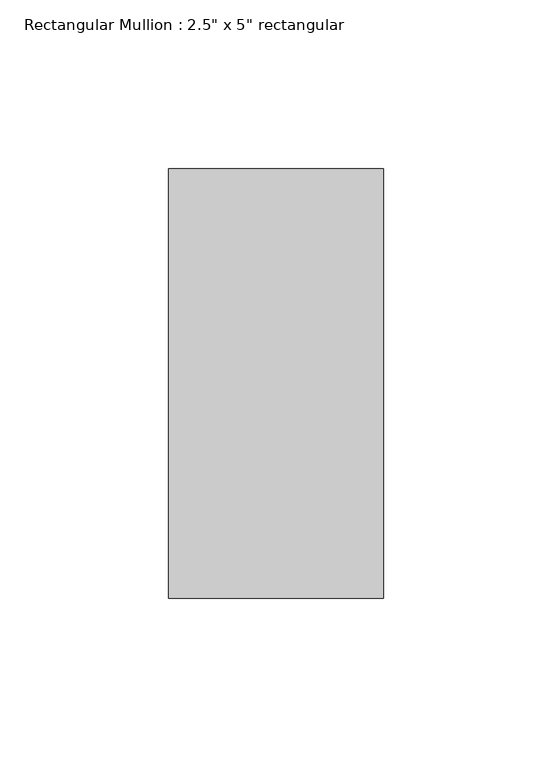
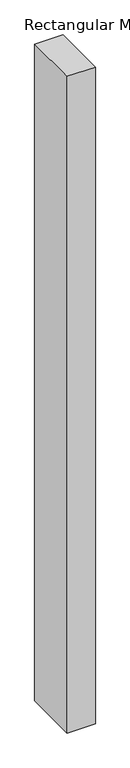
"""IFC4 building model written with IfcOpenShell, lengths in millimetres: member geometry."""

from ifc_helpers import new_model, si_unit, frame, origin, place, context, project, spatial, polyline, outline, extrude, source, transform, mapped, element, save


def member_2ac6f7d4(model_context):
    return source(origin(), model_context, "Body", "SweptSolid", [
        extrude(outline(polyline([(0.0, 63.5), (0.0, -63.5), (-63.5, -63.5), (-63.5, 63.5), (0.0, 63.5)])), frame((0.0, 0.0, -1566.9800364), z_axis=(0.0, 0.0, 1.0), x_axis=(1.0, 0.0, 0.0)), (0.0, 0.0, 1.0), 1566.9800364),
    ])


if __name__ == "__main__":
    model = new_model("IFC4")
    model_context = context("Model", 3, world=origin())
    ifc_project = project(units=[si_unit("LENGTHUNIT", "METRE", prefix="MILLI")], contexts=[model_context])
    site = spatial("IfcSite", under=ifc_project)
    building = spatial("IfcBuilding", under=site)
    placement = place(None, origin())
    member_shape = member_2ac6f7d4(model_context)
    element("IfcMember", 1, ObjectType="Rectangular Mullion : 2.5\" x 5\" rectangular", at=placement, inside=building, context=model_context, shape_type="MappedRepresentation", body=[
        mapped(member_shape, transform((0.0, 0.0, 0.0), x_axis=(1.0, 0.0, 0.0), y_axis=(0.0, 1.0, 0.0), z_axis=(0.0, 0.0, 1.0))),
    ])
    save(model, "model.ifc")

# Revit data of these elements
# Type "Rectangular Mullion : 2.5\" x 5\" rectangular"
#   built-in parameter 1007304 = 0.416667 (stored number, unit not read)
#   built-in parameter 1007301 = 0.104167 (stored number, unit not read)
#   built-in parameter 1007300 = 0.104167 (stored number, unit not read)
# Element 1 (IfcMember, "Rectangular Mullion : 2.5\" x 5\" rectangular")
#   Materials on its faces: "Aluminum"
# Materials
#   "Aluminum": class "Metal", colour RGB 247 247 247, transparency 0, Description = "Aluminum 6061", Cost = 0
